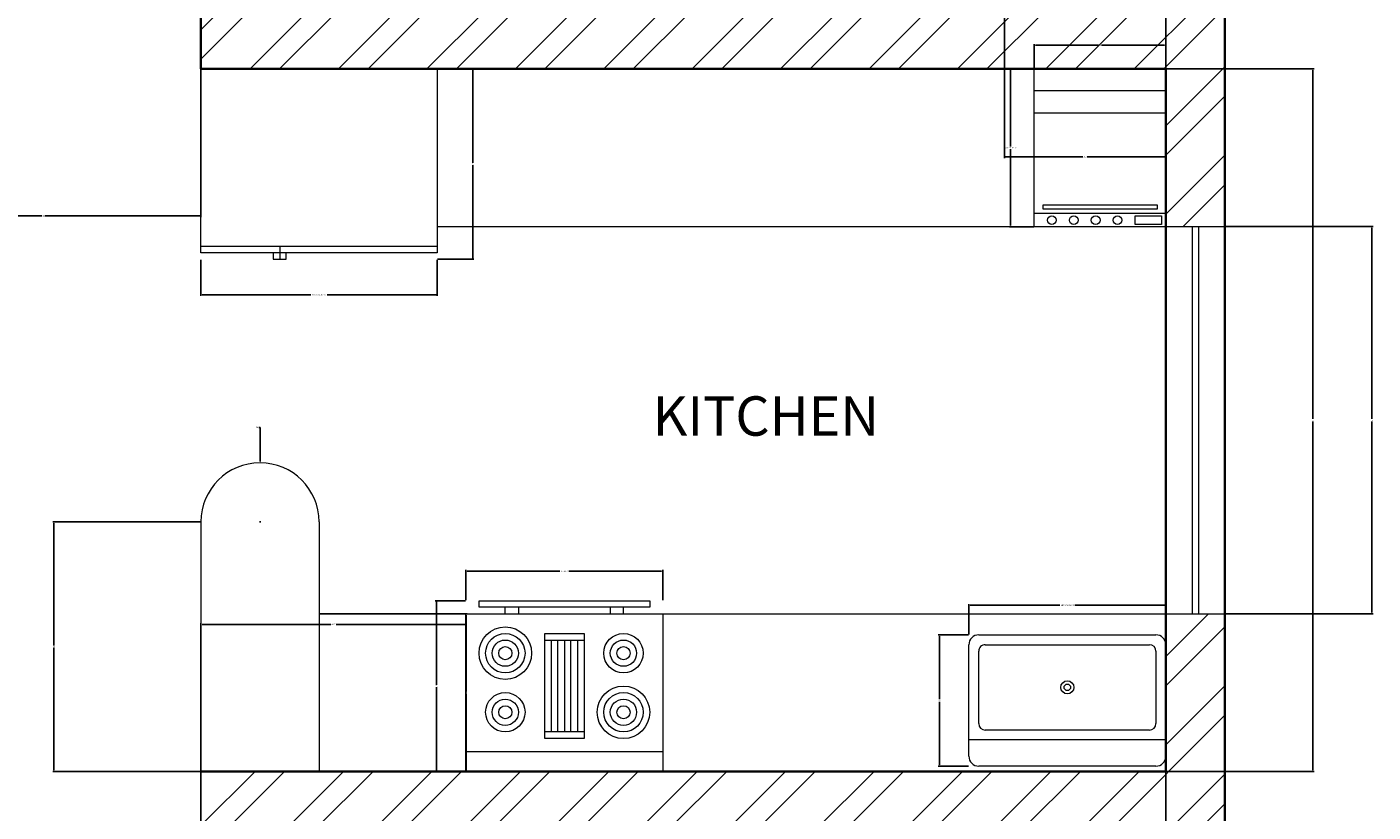
# Model space of a CAD drawing. Units: inches. Extents: x 3449 to 3843, y 1566 to 2054.
# Tile 5 of 8: x 3638 to 3843, y 1726 to 1846. Entities that reach past the tile are written whole.
import ezdxf

# ---------------------------------------------------------------- set-up
doc = ezdxf.new("R2010")
doc.units = ezdxf.units.IN
for name, color, linetype, lineweight in [('A-ANNO-DIMS', 2, 'Continuous', 18), ('A-AREA-IDEN', 7, 'Continuous', 25), ('A-EQPM', 8, 'Continuous', 18), ('A-FLOR-CASE', 7, 'Continuous', 20), ('A-GLAZ', 5, 'Continuous', 18), ('A-WALL', 7, 'Continuous', 35), ('A-WALL-PATT', 251, 'Continuous', 13), ('Сантехника', 7, 'Continuous', 18)]:
    doc.layers.add(name, color=color, linetype=linetype, lineweight=lineweight)
doc.styles.get("Standard").update_dxf_attribs({"font": 'arial.ttf'})
doc.dimstyles.get("Standard").update_dxf_attribs({"dimtxt": 0.18, "dimasz": 0.18, "dimexe": 0.18, "dimexo": 0.0625, "dimgap": 0.09, "dimtad": 0, "dimtih": 1, "dimtoh": 1, "dimdec": 4, "dimzin": 0, "dimdsep": 46, "dimtxsty": 'Standard', "dimcen": 0.09, "dimadec": 0, "dimazin": 0, "dimtfac": 1, "dimtdec": 4, "dimtofl": 0, "dimtmove": 0, "dimatfit": 3, "dimfxl": 1, "dimtolj": 1, "dimtzin": 0, "dimarcsym": 0})

# ---------------------------------------------------------------- blocks, each defined once
blk = doc.blocks.new('Range-Oven - 30 in top')
for p, q in [((0, -3), (30, -3)), ((12, -6), (18, -6)), ((13, -20), (13, -6)), ((14, -6), (14, -20)), ((15, -20), (15, -6)), ((16, -6), (16, -20)), ((17, -20), (17, -6)), ((18, -20), (12, -20)), ((6, -24), (6, -25)), ((8, -25), (8, -24)), ((22, -25), (22, -24)), ((24, -24), (24, -25))]:
    blk.add_line(p, q)
for points in [[(0, -24), (0, 0), (30, 0), (30, -24)], [(12, -21), (12, -5), (18, -5), (18, -21)], [(2, -26), (2, -25), (28, -25), (28, -26)]]:
    blk.add_lwpolyline(points, close=True)
for centre, radius in [((6, -9), 4), ((6, -9), 3), ((24, -9), 3), ((6, -9), 2), ((6, -9), 1), ((24, -9), 2), ((24, -9), 1), ((24, -18), 4), ((6, -18), 3), ((6, -18), 2), ((24, -18), 3), ((24, -18), 2), ((6, -18), 1), ((24, -18), 1)]:
    blk.add_circle(centre, radius)
blk = doc.blocks.new('Refrigerator-2 door - 36 in top')
for p, q in [((0, -26.999999), (36, -26.999999)), ((11, -27.999999), (11, -28.999999)), ((12, -26.999999), (12, -28.999999)), ((13, -28.999999), (13, -27.999999)), ((11, -28.999999), (13, -28.999999))]:
    blk.add_line(p, q)
blk.add_lwpolyline([(0, -27.999999), (0, 0), (36, 0), (36, -27.999999)], close=True)
blk = doc.blocks.new('Range-Oven - 30 in front')
for p, q in [((0, 33.00005), (30, 33.00005)), ((30, 10), (0, 10)), ((0, 5), (30, 5))]:
    blk.add_line(p, q)
for points in [[(0, 0), (0, 36.00005), (30, 36.00005), (30, 0)], [(1, 33.50005), (1, 35.50005), (7, 35.50005), (7, 33.50005)], [(2, 31.00005), (2, 32.00005), (28, 32.00005), (28, 31.00005)]]:
    blk.add_lwpolyline(points, close=True)
for centre in [(11, 34.50005), (16, 34.50005), (21, 34.50005), (26, 34.50005)]:
    blk.add_circle(centre, 1)
blk = doc.blocks.new('Sink-single - 30 in top')
blk.add_line((-15, -3.999996), (15, -3.999996))
for points in [[(-13.5, 0), (13.5, 0)], [(-15, -18.499996), (-15, -1.5)], [(15, -1.5), (15, -18.499996)], [(-12.5, -5.499996), (12.5, -5.499996)], [(-13.5, -17.499996), (-13.5, -6.499996)], [(13.5, -6.499996), (13.5, -17.499996)], [(13.5, -19.999996), (-13.5, -19.999996)], [(12.5, -18.499996), (-12.5, -18.499996)]]:
    blk.add_lwpolyline(points)
for radius in [1, 0.5]:
    blk.add_circle((0, -11.999996), radius)
for centre, radius, start, end in [((-13.5, -1.5), 1.5, 90, 180), ((13.5, -1.5), 1.5, 0, 90), ((-12.5, -6.499996), 1, 90, 180), ((12.5, -6.499996), 1, 0, 90), ((-12.5, -17.499996), 1, 180, 270), ((12.5, -17.499996), 1, 270, 0), ((-13.5, -18.499996), 1.5, 180, 270), ((13.5, -18.499996), 1.5, 270, 0)]:
    blk.add_arc(centre, radius, start, end)
blk = doc.blocks.new('*D66')
at = {"layer": 'A-ANNO-DIMS', "color": 0, "lineweight": -2, "transparency": 16777216}
for p, q in [((3704.46, 1758.68), (3704.46, 1763.29)), ((3704.64, 1763.11), (3718.76, 1763.11)), ((3734.28, 1763.11), (3720.16, 1763.11)), ((3734.46, 1758.68), (3734.46, 1763.29))]:
    blk.add_line(p, q, dxfattribs=at)
at = {"layer": 'A-ANNO-DIMS', "color": 0, "transparency": 16777216}
for points in [[(3704.64, 1763.14), (3704.64, 1763.08), (3704.46, 1763.11)], [(3734.28, 1763.14), (3734.28, 1763.08), (3734.46, 1763.11)]]:
    blk.add_solid(points, dxfattribs=at)
at = {"layer": 'Defpoints', "color": 0, "transparency": 16777216}
for p in [(3704.46, 1763.11), (3704.46, 1758.61), (3734.46, 1758.61)]:
    blk.add_point(p, dxfattribs=at)
at = {"layer": 'A-ANNO-DIMS', "color": 0, "transparency": 16777216, "insert": (3719.46, 1763.11), "char_height": 0.18, "attachment_point": 5}
blk.add_mtext('\\A1;RANGE 30', dxfattribs=at)
blk = doc.blocks.new('*D67')
at = {"layer": 'A-ANNO-DIMS', "color": 0, "lineweight": -2, "transparency": 16777216}
for p, q in [((3704.4, 1758.61), (3699.78, 1758.61)), ((3699.96, 1758.43), (3699.96, 1745.8)), ((3699.96, 1732.79), (3699.96, 1745.43)), ((3704.4, 1732.61), (3699.78, 1732.61))]:
    blk.add_line(p, q, dxfattribs=at)
at = {"layer": 'A-ANNO-DIMS', "color": 0, "transparency": 16777216}
for points in [[(3699.93, 1758.43), (3699.99, 1758.43), (3699.96, 1758.61)], [(3699.93, 1732.79), (3699.99, 1732.79), (3699.96, 1732.61)]]:
    blk.add_solid(points, dxfattribs=at)
at = {"layer": 'Defpoints', "color": 0, "transparency": 16777216}
for p in [(3704.46, 1758.61), (3699.96, 1732.61), (3704.46, 1732.61)]:
    blk.add_point(p, dxfattribs=at)
at = {"layer": 'A-ANNO-DIMS', "color": 0, "transparency": 16777216, "insert": (3699.96, 1745.61), "char_height": 0.18, "attachment_point": 5}
blk.add_mtext('\\A1;26', dxfattribs=at)
blk = doc.blocks.new('*D68')
at = {"layer": 'A-ANNO-DIMS', "color": 0, "lineweight": -2, "transparency": 16777216}
for p, q in [((3664.09, 1810.55), (3664.09, 1805.03)), ((3700.09, 1810.55), (3700.09, 1805.03)), ((3664.27, 1805.21), (3680.84, 1805.21)), ((3699.91, 1805.21), (3683.34, 1805.21))]:
    blk.add_line(p, q, dxfattribs=at)
at = {"layer": 'A-ANNO-DIMS', "color": 0, "transparency": 16777216}
for points in [[(3664.27, 1805.24), (3664.27, 1805.18), (3664.09, 1805.21)], [(3699.91, 1805.24), (3699.91, 1805.18), (3700.09, 1805.21)]]:
    blk.add_solid(points, dxfattribs=at)
at = {"layer": 'Defpoints', "color": 0, "transparency": 16777216}
for p in [(3664.09, 1810.61), (3700.09, 1810.61), (3700.09, 1805.21)]:
    blk.add_point(p, dxfattribs=at)
at = {"layer": 'A-ANNO-DIMS', "color": 0, "transparency": 16777216, "insert": (3682.09, 1805.21), "char_height": 0.18, "attachment_point": 5}
blk.add_mtext('\\A1;REFRIGERATOR 36', dxfattribs=at)
blk = doc.blocks.new('*D69')
at = {"layer": 'A-ANNO-DIMS', "color": 0, "lineweight": -2, "transparency": 16777216}
for p, q in [((3700.15, 1839.61), (3705.67, 1839.61)), ((3705.49, 1839.43), (3705.49, 1825.3)), ((3705.49, 1810.79), (3705.49, 1824.93)), ((3700.15, 1810.61), (3705.67, 1810.61))]:
    blk.add_line(p, q, dxfattribs=at)
at = {"layer": 'A-ANNO-DIMS', "color": 0, "transparency": 16777216}
for points in [[(3705.46, 1839.43), (3705.52, 1839.43), (3705.49, 1839.61)], [(3705.46, 1810.79), (3705.52, 1810.79), (3705.49, 1810.61)]]:
    blk.add_solid(points, dxfattribs=at)
at = {"layer": 'Defpoints', "color": 0, "transparency": 16777216}
for p in [(3700.09, 1839.61), (3705.49, 1839.61), (3700.09, 1810.61)]:
    blk.add_point(p, dxfattribs=at)
at = {"layer": 'A-ANNO-DIMS', "color": 0, "transparency": 16777216, "insert": (3705.49, 1825.11), "char_height": 0.18, "attachment_point": 5}
blk.add_mtext('\\A1;29', dxfattribs=at)
blk = doc.blocks.new('*D70')
at = {"layer": 'A-ANNO-DIMS', "color": 0, "lineweight": -2, "transparency": 16777216}
for p, q in [((3790.99, 1839.61), (3787.26, 1839.61)), ((3787.44, 1839.43), (3787.44, 1827.77)), ((3787.44, 1815.75), (3787.44, 1827.41)), ((3790.99, 1815.57), (3787.26, 1815.57))]:
    blk.add_line(p, q, dxfattribs=at)
at = {"layer": 'A-ANNO-DIMS', "color": 0, "transparency": 16777216}
for points in [[(3787.41, 1839.43), (3787.47, 1839.43), (3787.44, 1839.61)], [(3787.41, 1815.75), (3787.47, 1815.75), (3787.44, 1815.57)]]:
    blk.add_solid(points, dxfattribs=at)
at = {"layer": 'Defpoints', "color": 0, "transparency": 16777216}
for p in [(3791.05, 1839.61), (3787.44, 1815.57), (3791.05, 1815.57)]:
    blk.add_point(p, dxfattribs=at)
at = {"layer": 'A-ANNO-DIMS', "color": 0, "transparency": 16777216, "insert": (3787.44, 1827.59), "char_height": 0.18, "attachment_point": 5}
blk.add_mtext('\\A1;OVEN FRONT 24', dxfattribs=at)
blk = doc.blocks.new('*D71')
at = {"layer": 'A-ANNO-DIMS', "color": 0, "lineweight": -2, "transparency": 16777216}
for p, q in [((3791.05, 1839.68), (3791.05, 1843.4)), ((3791.23, 1843.22), (3800.85, 1843.22)), ((3810.91, 1843.22), (3801.29, 1843.22)), ((3811.09, 1839.68), (3811.09, 1843.4))]:
    blk.add_line(p, q, dxfattribs=at)
at = {"layer": 'A-ANNO-DIMS', "color": 0, "transparency": 16777216}
for points in [[(3791.23, 1843.25), (3791.23, 1843.19), (3791.05, 1843.22)], [(3810.91, 1843.25), (3810.91, 1843.19), (3811.09, 1843.22)]]:
    blk.add_solid(points, dxfattribs=at)
at = {"layer": 'Defpoints', "color": 0, "transparency": 16777216}
for p in [(3791.05, 1843.22), (3791.05, 1839.61), (3811.09, 1839.61)]:
    blk.add_point(p, dxfattribs=at)
at = {"layer": 'A-ANNO-DIMS', "color": 0, "transparency": 16777216, "insert": (3801.07, 1843.22), "char_height": 0.18, "attachment_point": 5}
blk.add_mtext('\\A1;20', dxfattribs=at)
blk = doc.blocks.new('*D74')
at = {"layer": 'A-ANNO-DIMS', "color": 0, "lineweight": -2, "transparency": 16777216}
for p, q in [((3781.09, 1753.48), (3781.09, 1758.09)), ((3781.27, 1757.91), (3794.96, 1757.91)), ((3810.91, 1757.91), (3797.22, 1757.91)), ((3811.09, 1753.48), (3811.09, 1758.09))]:
    blk.add_line(p, q, dxfattribs=at)
at = {"layer": 'A-ANNO-DIMS', "color": 0, "transparency": 16777216}
for points in [[(3781.27, 1757.94), (3781.27, 1757.88), (3781.09, 1757.91)], [(3810.91, 1757.94), (3810.91, 1757.88), (3811.09, 1757.91)]]:
    blk.add_solid(points, dxfattribs=at)
at = {"layer": 'Defpoints', "color": 0, "transparency": 16777216}
for p in [(3781.09, 1757.91), (3781.09, 1753.41), (3811.09, 1753.41)]:
    blk.add_point(p, dxfattribs=at)
at = {"layer": 'A-ANNO-DIMS', "color": 0, "transparency": 16777216, "insert": (3796.09, 1757.91), "char_height": 0.18, "attachment_point": 5}
blk.add_mtext('\\A1;KITCHEN SINK 30', dxfattribs=at)
blk = doc.blocks.new('*D75')
at = {"layer": 'A-ANNO-DIMS', "color": 0, "lineweight": -2, "transparency": 16777216}
for p, q in [((3781.03, 1753.41), (3776.41, 1753.41)), ((3776.59, 1753.23), (3776.59, 1743.6)), ((3776.59, 1733.59), (3776.59, 1743.23)), ((3781.03, 1733.41), (3776.41, 1733.41))]:
    blk.add_line(p, q, dxfattribs=at)
at = {"layer": 'A-ANNO-DIMS', "color": 0, "transparency": 16777216}
for points in [[(3776.56, 1753.23), (3776.62, 1753.23), (3776.59, 1753.41)], [(3776.56, 1733.59), (3776.62, 1733.59), (3776.59, 1733.41)]]:
    blk.add_solid(points, dxfattribs=at)
at = {"layer": 'Defpoints', "color": 0, "transparency": 16777216}
for p in [(3781.09, 1753.41), (3776.59, 1733.41), (3781.09, 1733.41)]:
    blk.add_point(p, dxfattribs=at)
at = {"layer": 'A-ANNO-DIMS', "color": 0, "transparency": 16777216, "insert": (3776.59, 1743.41), "char_height": 0.18, "attachment_point": 5}
blk.add_mtext('\\A1;20', dxfattribs=at)
blk = doc.blocks.new('*D91')
at = {"layer": 'A-ANNO-DIMS', "color": 0, "lineweight": -2, "transparency": 16777216}
for p, q in [((3664.09, 1732.55), (3664.09, 1710.03)), ((3811.09, 1732.55), (3811.09, 1710.03)), ((3664.27, 1710.21), (3737.31, 1710.21)), ((3810.91, 1710.21), (3737.87, 1710.21))]:
    blk.add_line(p, q, dxfattribs=at)
at = {"layer": 'A-ANNO-DIMS', "color": 0, "transparency": 16777216}
for points in [[(3664.27, 1710.24), (3664.27, 1710.18), (3664.09, 1710.21)], [(3810.91, 1710.24), (3810.91, 1710.18), (3811.09, 1710.21)]]:
    blk.add_solid(points, dxfattribs=at)
at = {"layer": 'Defpoints', "color": 0, "transparency": 16777216}
for p in [(3664.09, 1732.61), (3811.09, 1732.61), (3664.09, 1710.21)]:
    blk.add_point(p, dxfattribs=at)
at = {"layer": 'A-ANNO-DIMS', "color": 0, "transparency": 16777216, "insert": (3737.59, 1710.21), "char_height": 0.18, "attachment_point": 5}
blk.add_mtext('\\A1;147', dxfattribs=at)
blk = doc.blocks.new('*D92')
at = {"layer": 'A-ANNO-DIMS', "color": 0, "lineweight": -2, "transparency": 16777216}
for p, q in [((3811.15, 1839.61), (3833.67, 1839.61)), ((3833.49, 1839.43), (3833.49, 1786.3)), ((3833.49, 1732.79), (3833.49, 1785.93)), ((3811.15, 1732.61), (3833.67, 1732.61))]:
    blk.add_line(p, q, dxfattribs=at)
at = {"layer": 'A-ANNO-DIMS', "color": 0, "transparency": 16777216}
for points in [[(3833.46, 1839.43), (3833.52, 1839.43), (3833.49, 1839.61)], [(3833.46, 1732.79), (3833.52, 1732.79), (3833.49, 1732.61)]]:
    blk.add_solid(points, dxfattribs=at)
at = {"layer": 'Defpoints', "color": 0, "transparency": 16777216}
for p in [(3811.09, 1839.61), (3811.09, 1732.61), (3833.49, 1732.61)]:
    blk.add_point(p, dxfattribs=at)
at = {"layer": 'A-ANNO-DIMS', "color": 0, "transparency": 16777216, "insert": (3833.49, 1786.11), "char_height": 0.18, "attachment_point": 5}
blk.add_mtext('\\A1;107', dxfattribs=at)
blk = doc.blocks.new('*D93')
at = {"layer": 'A-ANNO-DIMS', "color": 0, "lineweight": -2, "transparency": 16777216}
for p, q in [((3820.15, 1815.61), (3842.67, 1815.61)), ((3842.49, 1815.43), (3842.49, 1786.3)), ((3842.49, 1756.79), (3842.49, 1785.93)), ((3820.15, 1756.61), (3842.67, 1756.61))]:
    blk.add_line(p, q, dxfattribs=at)
at = {"layer": 'A-ANNO-DIMS', "color": 0, "transparency": 16777216}
for points in [[(3842.46, 1815.43), (3842.52, 1815.43), (3842.49, 1815.61)], [(3842.46, 1756.79), (3842.52, 1756.79), (3842.49, 1756.61)]]:
    blk.add_solid(points, dxfattribs=at)
at = {"layer": 'Defpoints', "color": 0, "transparency": 16777216}
for p in [(3820.09, 1815.61), (3820.09, 1756.61), (3842.49, 1756.61)]:
    blk.add_point(p, dxfattribs=at)
at = {"layer": 'A-ANNO-DIMS', "color": 0, "transparency": 16777216, "insert": (3842.49, 1786.11), "char_height": 0.18, "attachment_point": 5}
blk.add_mtext('\\A1;59', dxfattribs=at)
blk = doc.blocks.new('*D94')
at = {"layer": 'A-ANNO-DIMS', "color": 0, "lineweight": -2, "transparency": 16777216}
for p, q in [((3616.09, 1839.55), (3616.09, 1817.03)), ((3664.09, 1839.55), (3664.09, 1817.03)), ((3616.27, 1817.21), (3639.87, 1817.21)), ((3663.91, 1817.21), (3640.31, 1817.21))]:
    blk.add_line(p, q, dxfattribs=at)
at = {"layer": 'A-ANNO-DIMS', "color": 0, "transparency": 16777216}
for points in [[(3616.27, 1817.24), (3616.27, 1817.18), (3616.09, 1817.21)], [(3663.91, 1817.24), (3663.91, 1817.18), (3664.09, 1817.21)]]:
    blk.add_solid(points, dxfattribs=at)
at = {"layer": 'Defpoints', "color": 0, "transparency": 16777216}
for p in [(3616.09, 1839.61), (3664.09, 1839.61), (3616.09, 1817.21)]:
    blk.add_point(p, dxfattribs=at)
at = {"layer": 'A-ANNO-DIMS', "color": 0, "transparency": 16777216, "insert": (3640.09, 1817.21), "char_height": 0.18, "attachment_point": 5}
blk.add_mtext('\\A1;48', dxfattribs=at)
blk = doc.blocks.new('*D117')
at = {"layer": 'A-ANNO-DIMS', "color": 0, "lineweight": -2, "transparency": 16777216}
for p, q in [((3664.09, 1732.68), (3664.09, 1755.19)), ((3664.27, 1755.01), (3683.88, 1755.01)), ((3704.28, 1755.01), (3684.67, 1755.01)), ((3704.46, 1732.68), (3704.46, 1755.19))]:
    blk.add_line(p, q, dxfattribs=at)
at = {"layer": 'A-ANNO-DIMS', "color": 0, "transparency": 16777216}
for points in [[(3664.27, 1755.04), (3664.27, 1754.98), (3664.09, 1755.01)], [(3704.28, 1755.04), (3704.28, 1754.98), (3704.46, 1755.01)]]:
    blk.add_solid(points, dxfattribs=at)
at = {"layer": 'Defpoints', "color": 0, "transparency": 16777216}
for p in [(3704.46, 1755.01), (3664.09, 1732.61), (3704.46, 1732.61)]:
    blk.add_point(p, dxfattribs=at)
at = {"layer": 'A-ANNO-DIMS', "color": 0, "transparency": 16777216, "insert": (3684.27, 1755.01), "char_height": 0.18, "attachment_point": 5}
blk.add_mtext('\\A1;40.37', dxfattribs=at)
blk = doc.blocks.new('*D118')
at = {"layer": 'A-ANNO-DIMS', "color": 0, "lineweight": -2, "transparency": 16777216}
for p, q in [((3682.15, 1756.61), (3704.67, 1756.61)), ((3704.49, 1756.43), (3704.49, 1744.79)), ((3704.49, 1732.79), (3704.49, 1744.43)), ((3682.15, 1732.61), (3704.67, 1732.61))]:
    blk.add_line(p, q, dxfattribs=at)
at = {"layer": 'A-ANNO-DIMS', "color": 0, "transparency": 16777216}
for points in [[(3704.46, 1756.43), (3704.52, 1756.43), (3704.49, 1756.61)], [(3704.46, 1732.79), (3704.52, 1732.79), (3704.49, 1732.61)]]:
    blk.add_solid(points, dxfattribs=at)
at = {"layer": 'Defpoints', "color": 0, "transparency": 16777216}
for p in [(3682.09, 1756.61), (3682.09, 1732.61), (3704.49, 1732.61)]:
    blk.add_point(p, dxfattribs=at)
at = {"layer": 'A-ANNO-DIMS', "color": 0, "transparency": 16777216, "insert": (3704.49, 1744.61), "char_height": 0.18, "attachment_point": 5}
blk.add_mtext('\\A1;24', dxfattribs=at)
blk = doc.blocks.new('*D123')
at = {"layer": 'A-ANNO-DIMS', "color": 0, "lineweight": -2, "transparency": 16777216}
for p, q in [((3664.03, 1770.61), (3641.51, 1770.61)), ((3641.69, 1770.43), (3641.69, 1751.8)), ((3641.69, 1732.79), (3641.69, 1751.43)), ((3664.03, 1732.61), (3641.51, 1732.61))]:
    blk.add_line(p, q, dxfattribs=at)
at = {"layer": 'A-ANNO-DIMS', "color": 0, "transparency": 16777216}
for points in [[(3641.66, 1770.43), (3641.72, 1770.43), (3641.69, 1770.61)], [(3641.66, 1732.79), (3641.72, 1732.79), (3641.69, 1732.61)]]:
    blk.add_solid(points, dxfattribs=at)
at = {"layer": 'Defpoints', "color": 0, "transparency": 16777216}
for p in [(3641.69, 1770.61), (3664.09, 1770.61), (3664.09, 1732.61)]:
    blk.add_point(p, dxfattribs=at)
at = {"layer": 'A-ANNO-DIMS', "color": 0, "transparency": 16777216, "insert": (3641.69, 1751.61), "char_height": 0.18, "attachment_point": 5}
blk.add_mtext('\\A1;38', dxfattribs=at)
blk = doc.blocks.new('*D124')
at = {"layer": 'A-ANNO-DIMS', "color": 0, "lineweight": -2, "transparency": 16777216}
for p, q in [((3786.49, 1848.55), (3786.49, 1826.03)), ((3811.09, 1848.55), (3811.09, 1826.03)), ((3786.67, 1826.21), (3798.46, 1826.21)), ((3810.91, 1826.21), (3799.11, 1826.21))]:
    blk.add_line(p, q, dxfattribs=at)
at = {"layer": 'A-ANNO-DIMS', "color": 0, "transparency": 16777216}
for points in [[(3786.67, 1826.24), (3786.67, 1826.18), (3786.49, 1826.21)], [(3810.91, 1826.24), (3810.91, 1826.18), (3811.09, 1826.21)]]:
    blk.add_solid(points, dxfattribs=at)
at = {"layer": 'Defpoints', "color": 0, "transparency": 16777216}
for p in [(3786.49, 1848.61), (3811.09, 1848.61), (3786.49, 1826.21)]:
    blk.add_point(p, dxfattribs=at)
at = {"layer": 'A-ANNO-DIMS', "color": 0, "transparency": 16777216, "insert": (3798.79, 1826.21), "char_height": 0.18, "attachment_point": 5}
blk.add_mtext('\\A1;24.6', dxfattribs=at)
blk = doc.blocks.new('*D126')
at = {"layer": 'A-ANNO-DIMS', "color": 0, "lineweight": -2, "transparency": 16777216}
for p, q in [((3672.91, 1785.01), (3673.09, 1785.01)), ((3673.09, 1785.01), (3673.09, 1779.79)), ((3673, 1770.61), (3673.18, 1770.61)), ((3673.09, 1770.52), (3673.09, 1770.7))]:
    blk.add_line(p, q, dxfattribs=at)
at = {"layer": 'A-ANNO-DIMS', "color": 0, "transparency": 16777216}
blk.add_solid([(3673.12, 1779.79), (3673.06, 1779.79), (3673.09, 1779.61)], dxfattribs=at)
at = {"layer": 'Defpoints', "color": 0, "transparency": 16777216}
for p in [(3673.09, 1779.61), (3673.09, 1770.61)]:
    blk.add_point(p, dxfattribs=at)
at = {"layer": 'A-ANNO-DIMS', "color": 0, "transparency": 16777216, "insert": (3672.67, 1785.01), "char_height": 0.18, "attachment_point": 5}
blk.add_mtext('\\A1;R9', dxfattribs=at)

msp = doc.modelspace()

# ---------------------------------------------------------------- hatches: boundary and pattern name
at = {"layer": 'A-WALL-PATT'}
h = msp.add_hatch(dxfattribs=at)
h.set_pattern_fill('ANSI32', color=256)
edge = h.paths.add_edge_path()
edge.add_line((3481.088, 2022.6144), (3508.088, 2022.6144))
edge.add_line((3508.088, 2022.6144), (3508.088, 2031.6144))
edge.add_line((3508.088, 2031.6144), (3472.088, 2031.6144))
edge.add_line((3472.088, 2031.6144), (3472.088, 1779.6144))
edge.add_line((3472.088, 1779.6144), (3481.088, 1779.6144))
edge.add_line((3481.088, 1779.6144), (3481.088, 1839.6144))
edge.add_line((3481.088, 1839.6144), (3571.088, 1839.6144))
edge.add_line((3571.088, 1839.6144), (3571.088, 1824.3194))
edge.add_line((3571.088, 1824.3194), (3571.088, 1821.6144))
edge.add_line((3571.088, 1821.6144), (3580.088, 1821.6144))
edge.add_line((3580.088, 1821.6144), (3580.088, 1825.1908))
edge.add_ellipse((3580.1411, 1825.2442), major_axis=(0, 0.0754), ratio=0.99913951, start_angle=90, end_angle=135.183195, ccw=False)
edge.add_line((3580.0017, 1825.3196), (3580.0658, 1825.3196))
edge.add_line((3580.0658, 1825.3196), (3580.066, 1839.6365))
edge.add_line((3580.066, 1839.6365), (3616.088, 1839.6365))
edge.add_line((3616.088, 1839.6365), (3616.088, 1848.6144))
edge.add_line((3616.088, 1848.6144), (3610.088, 1848.6144))
edge.add_line((3610.088, 1848.6144), (3574.088, 1848.6144))
edge.add_line((3574.088, 1848.6144), (3481.088, 1848.6144))
edge.add_line((3481.088, 1848.6144), (3481.088, 1872.6144))
edge.add_line((3481.088, 1872.6144), (3481.088, 2022.6144))
h.paths.add_polyline_path([(3550.088, 1779.6144), (3616.088, 1779.6144), (3616.088, 1791.6144), (3505.088, 1791.6144), (3505.088, 1779.6144), (3541.088, 1779.6144), (3541.088, 1657.6144), (3481.088, 1657.6144), (3481.088, 1588.6144), (3496.088, 1588.6144), (3496.088, 1594.6144), (3496.088, 1597.6144), (3490.088, 1597.6144), (3490.088, 1648.6144), (3550.088, 1648.6144)])
h.paths.add_polyline_path([(3775.088, 1612.6144), (3766.088, 1612.6144), (3766.088, 1597.6144), (3536.088, 1597.6144), (3536.088, 1588.6144), (3775.088, 1588.6144)])
h.paths.add_polyline_path([(3820.088, 1756.6144), (3811.088, 1756.6144), (3811.088, 1732.6144), (3664.088, 1732.6144), (3664.088, 1723.6144), (3766.088, 1723.6144), (3766.088, 1708.6144), (3775.088, 1708.6144), (3775.088, 1723.6144), (3820.088, 1723.6144)])
h.paths.add_polyline_path([(3820.088, 1986.6144), (3745.088, 1986.6144), (3745.088, 2010.6144), (3664.088, 2010.6144), (3664.088, 1992.6144), (3652.088, 1992.6144), (3652.088, 1983.6144), (3664.088, 1983.6144), (3664.088, 1893.6144), (3648.793, 1893.6144), (3607.088, 1893.6144), (3607.088, 1884.6144), (3673.088, 1884.6144), (3673.088, 2001.6144), (3736.088, 2001.6144), (3736.088, 1977.6144), (3811.088, 1977.6144), (3811.088, 1949.1144), (3820.088, 1949.1144)])
h.paths.add_polyline_path([(3628.088, 1992.6144), (3616.088, 1992.6144), (3616.088, 2031.6144), (3580.088, 2031.6144), (3580.088, 2022.6144), (3607.088, 2022.6144), (3607.088, 1921.6144), (3613.088, 1921.6144), (3616.088, 1921.6144), (3616.088, 1983.6144), (3628.088, 1983.6144)])
h.paths.add_polyline_path([(3820.088, 1877.1144), (3811.088, 1877.1144), (3811.088, 1848.6144), (3664.088, 1848.6144), (3664.088, 1839.6144), (3700.088, 1839.6144), (3811.088, 1839.6144), (3811.088, 1815.6144), (3820.088, 1815.6144)])

# ---------------------------------------------------------------- linework, layer by layer
at = {"layer": 'A-FLOR-CASE'}
for p, q in [((3700.088, 1815.6144), (3820.088, 1815.6144)), ((3664.088, 1770.6144), (3664.088, 1713.6144)), ((3682.088, 1770.6144), (3682.088, 1732.6144)), ((3682.088, 1756.6144), (3820.088, 1756.6144))]:
    msp.add_line(p, q, dxfattribs=at)
msp.add_arc((3673.088, 1770.6144), 9, 0, 180, dxfattribs=at)
at = {"layer": 'A-GLAZ'}
for p, q in [((3815.088, 1815.6144), (3815.088, 1756.6144)), ((3816.088, 1815.6144), (3816.088, 1756.6144))]:
    msp.add_line(p, q, dxfattribs=at)
at = {"layer": 'A-WALL'}
for p, q in [((3820.088, 1949.1144), (3820.088, 1756.6144)), ((3664.088, 1848.6144), (3664.088, 1839.6144)), ((3664.088, 1839.6144), (3811.088, 1839.6144)), ((3811.088, 1839.6144), (3811.088, 1732.6144)), ((3820.088, 1756.6144), (3820.088, 1723.6144)), ((3664.088, 1732.6144), (3811.088, 1732.6144))]:
    msp.add_line(p, q, dxfattribs=at)

# ---------------------------------------------------------------- block references
at = {"layer": 'A-EQPM'}
msp.add_blockref('Refrigerator-2 door - 36 in top', (3664.088, 1839.6144), dxfattribs=at)
at = {"layer": 'A-EQPM', "xscale": 0.6680156577150776, "yscale": 0.6680156577150776, "zscale": 0.6680156577150776, "rotation": 180}
msp.add_blockref('Range-Oven - 30 in front', (3811.088, 1839.6144), dxfattribs=at)
at = {"layer": 'A-EQPM', "rotation": 180}
msp.add_blockref('Range-Oven - 30 in top', (3734.4602, 1732.6144), dxfattribs=at)
at = {"layer": 'Сантехника', "rotation": 180}
msp.add_blockref('Sink-single - 30 in top', (3796.088, 1733.4133), dxfattribs=at)

# ---------------------------------------------------------------- texts
at = {"layer": 'A-AREA-IDEN', "insert": (3732.918, 1789.7412), "char_height": 6, "attachment_point": 1}
msp.add_mtext_dynamic_manual_height_columns('KITCHEN', width=95.638287, gutter_width=12.5, heights=[0], dxfattribs=at)

# ---------------------------------------------------------------- dimensions: what is measured, and where the dimension line sits
at = {"layer": 'A-ANNO-DIMS'}
for base, p1, p2, angle, override, picture, middle in [((3786.488, 1826.2144), (3811.088, 1848.6144), (3786.488, 1848.6144), 180, {"dimdec": 1, "dimlfac": 1, "dimrnd": 0, "dimzin": 0, "dimdsep": 46, "dimlunit": 2}, '*D124', (3798.788, 1826.2144)), ((3791.0475, 1843.2217), (3811.088, 1839.6144), (3791.0475, 1839.6144), 180, {"dimdec": 0, "dimlfac": 1, "dimrnd": 0, "dimzin": 0, "dimdsep": 46, "dimlunit": 2}, '*D71', (3801.0678, 1843.2217)), ((3616.088, 1817.2144), (3664.088, 1839.6144), (3616.088, 1839.6144), 180, {"dimdec": 0, "dimlfac": 1, "dimrnd": 0, "dimzin": 0, "dimdsep": 46, "dimlunit": 2}, '*D94', (3640.088, 1817.2144)), ((3705.488, 1839.6144), (3700.088, 1810.6144), (3700.088, 1839.6144), 90, {"dimdec": 0, "dimlfac": 1, "dimrnd": 0, "dimzin": 0, "dimdsep": 46, "dimlunit": 2}, '*D69', (3705.488, 1825.1144)), ((3833.488, 1732.6144), (3811.088, 1839.6144), (3811.088, 1732.6144), 270, {"dimdec": 0, "dimlfac": 1, "dimrnd": 0, "dimzin": 0, "dimdsep": 46, "dimlunit": 2}, '*D92', (3833.488, 1786.1144)), ((3842.488, 1756.6144), (3820.088, 1815.6144), (3820.088, 1756.6144), 270, {"dimdec": 0, "dimlfac": 1, "dimrnd": 0, "dimzin": 0, "dimdsep": 46, "dimlunit": 2}, '*D93', (3842.488, 1786.1144)), ((3641.688, 1770.6144), (3664.088, 1732.6144), (3664.088, 1770.6144), 90, {"dimdec": 0, "dimlfac": 1, "dimrnd": 0, "dimzin": 0, "dimdsep": 46, "dimlunit": 2}, '*D123', (3641.688, 1751.6144)), ((3699.9602, 1732.6144), (3704.4602, 1758.6144), (3704.4602, 1732.6144), 270, {"dimdec": 0, "dimlfac": 1, "dimrnd": 0, "dimzin": 0, "dimdsep": 46, "dimlunit": 2}, '*D67', (3699.9602, 1745.6144)), ((3704.488, 1732.6144), (3682.088, 1756.6144), (3682.088, 1732.6144), 270, {"dimdec": 0, "dimlfac": 1, "dimrnd": 0, "dimzin": 0, "dimdsep": 46, "dimlunit": 2}, '*D118', (3704.488, 1744.6144)), ((3776.588, 1733.4133), (3781.088, 1753.4133), (3781.088, 1733.4133), 270, {"dimdec": 0, "dimlfac": 1, "dimrnd": 0, "dimzin": 0, "dimdsep": 46, "dimlunit": 2}, '*D75', (3776.588, 1743.4133)), ((3664.088, 1710.2144), (3811.088, 1732.6144), (3664.088, 1732.6144), 180, {"dimdec": 0, "dimlfac": 1, "dimrnd": 0, "dimzin": 0, "dimdsep": 46, "dimlunit": 2}, '*D91', (3737.588, 1710.2144))]:
    dim = msp.add_linear_dim(base=base, p1=p1, p2=p2, angle=angle, dimstyle='Standard', override=override, dxfattribs=at)
    dim.commit()
    dim.dimension.update_dxf_attribs({"geometry": picture, "text_midpoint": middle})
for base, p1, p2, angle, text, picture, middle in [((3787.4403, 1815.5658), (3791.0475, 1839.6144), (3791.0475, 1815.5658), 270, 'OVEN FRONT <>', '*D70', (3787.4403, 1827.5901)), ((3704.4602, 1763.1144), (3734.4602, 1758.6144), (3704.4602, 1758.6144), 180, 'RANGE <>', '*D66', (3719.4602, 1763.1144)), ((3781.088, 1757.9133), (3811.088, 1753.4133), (3781.088, 1753.4133), 180, 'KITCHEN SINK <>', '*D74', (3796.088, 1757.9133))]:
    dim = msp.add_linear_dim(base=base, p1=p1, p2=p2, angle=angle, text=text, dimstyle='Standard', override={"dimdec": 0, "dimlfac": 1, "dimrnd": 0, "dimzin": 0, "dimdsep": 46, "dimlunit": 2}, dxfattribs=at)
    dim.commit()
    dim.dimension.update_dxf_attribs({"geometry": picture, "text_midpoint": middle})
dim = msp.add_linear_dim(base=(3700.088, 1805.2144), p1=(3664.088, 1810.6144), p2=(3700.088, 1810.6144), text='REFRIGERATOR <>', dimstyle='Standard', override={"dimdec": 0, "dimlfac": 1, "dimrnd": 0, "dimzin": 0, "dimdsep": 46, "dimlunit": 2}, dxfattribs=at)
dim.commit()
dim.dimension.update_dxf_attribs({"geometry": '*D68', "text_midpoint": (3682.088, 1805.2144)})
dim = msp.add_radius_dim(center=(3673.088, 1770.6144), mpoint=(3673.088, 1779.6144), dimstyle='Standard', override={"dimdec": 0, "dimlfac": 1, "dimrnd": 0, "dimzin": 0, "dimdsep": 46, "dimlunit": 2}, dxfattribs=at)
dim.commit()
dim.dimension.update_dxf_attribs({"geometry": '*D126', "text_midpoint": (3672.6727, 1785.0144), "dimtype": 164})
dim = msp.add_linear_dim(base=(3704.4602, 1755.0144), p1=(3664.088, 1732.6144), p2=(3704.4602, 1732.6144), dimstyle='Standard', override={"dimdec": 2, "dimlfac": 1, "dimrnd": 0, "dimzin": 0, "dimdsep": 46, "dimlunit": 2}, dxfattribs=at)
dim.commit()
dim.dimension.update_dxf_attribs({"geometry": '*D117', "text_midpoint": (3684.2741, 1755.0144)})

doc.saveas('drawing.dxf')
